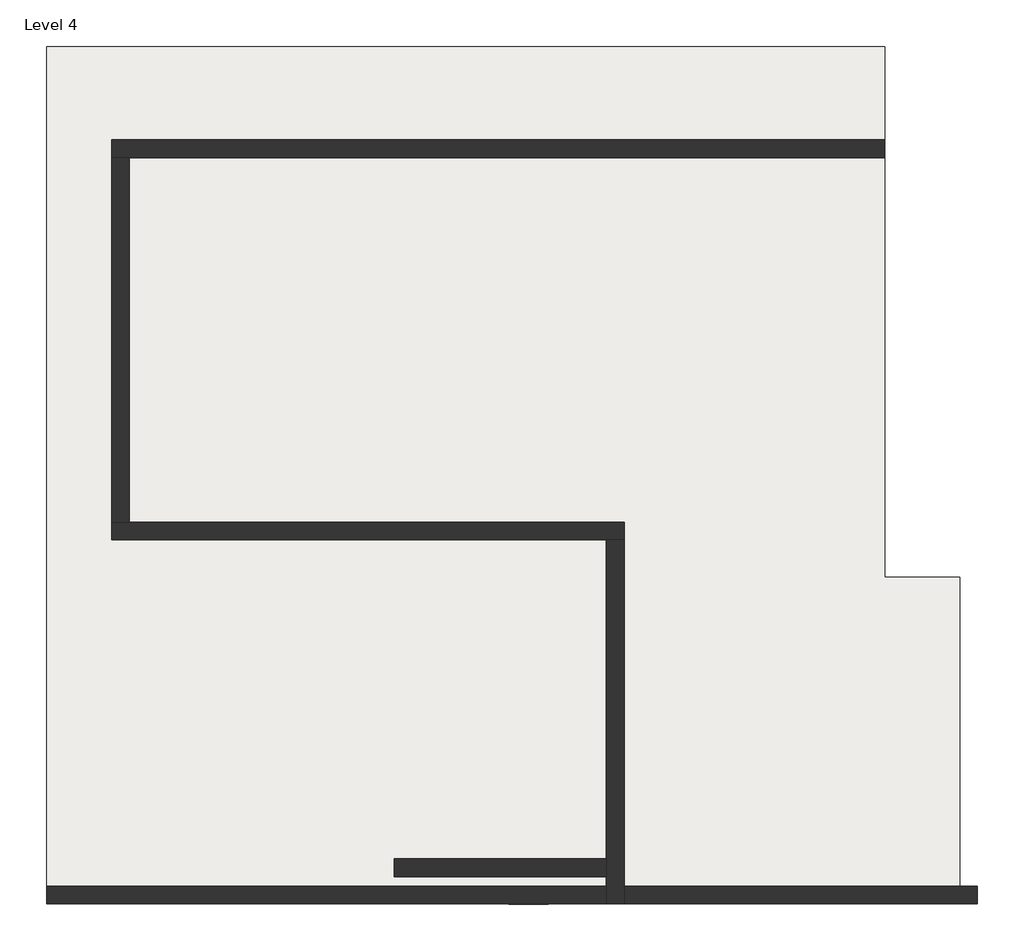
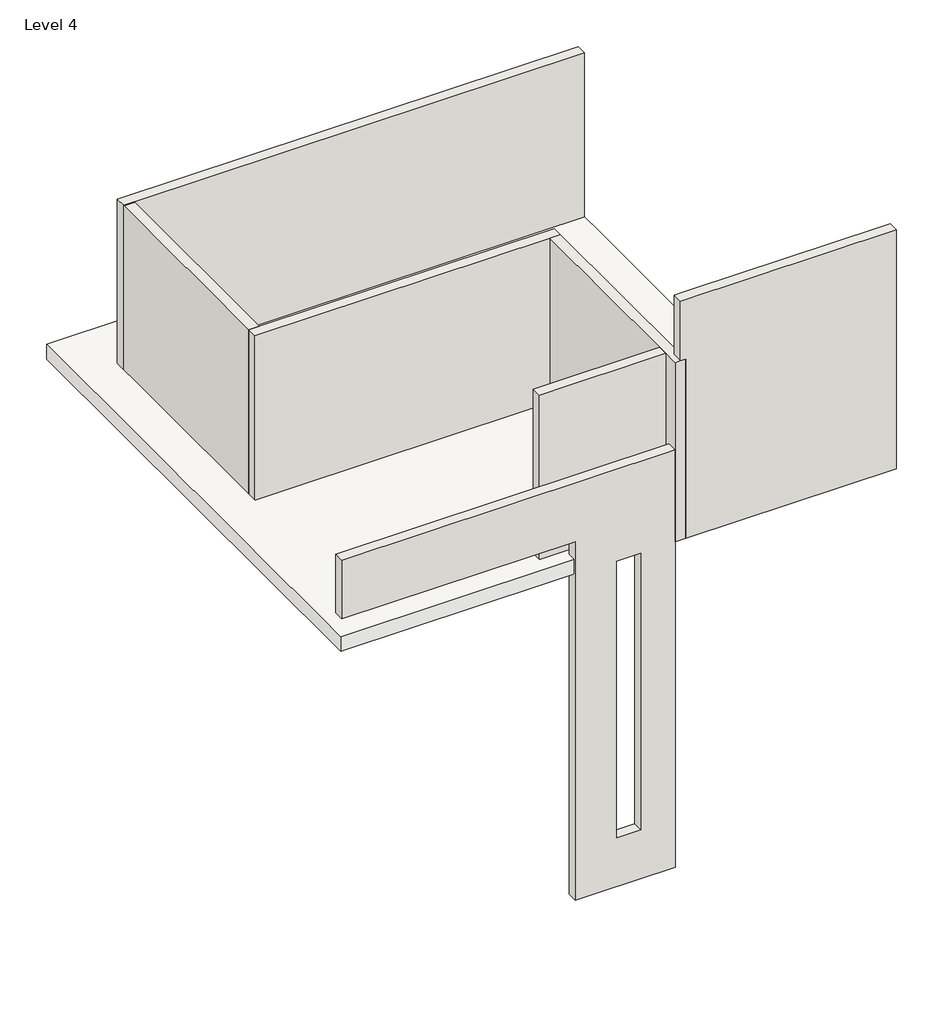
# One storey: 7 walls, 1 roof.
"""IFC4 building model written with IfcOpenShell, lengths in millimetres."""

from ifc_helpers import new_model, si_unit, frame, origin, place, context, project, spatial, polyline, outline, extrude, faceted_brep, element, save

model = new_model("IFC4")

# Units and contexts
model_context = context("Model", 3, world=origin())
ifc_project = project(units=[si_unit("LENGTHUNIT", "METRE", prefix="MILLI")], contexts=[model_context])

# Site, building, storey
site = spatial("IfcSite", under=ifc_project)
building = spatial("IfcBuilding", under=site)
storey = spatial("IfcBuildingStorey", under=building, Name="Level 4", Elevation=10972.8)

# Roof
placement = place(None, origin())
element("IfcRoof", 1, ObjectType="Generic - 12\"", at=placement, inside=storey, context=model_context, shape_type="SweptSolid", body=[
    extrude(outline(polyline([(-10862.1012689, 11214.3911137), (-1224.1821198, 11214.3911137), (-1224.1821198, 5111.80098), (-360.5821198, 5111.80098), (-360.5821198, 1387.3881635), (-10862.1012689, 1387.3881635), (-10862.1012689, 11214.3911137)])), frame((0.0, 0.0, 10972.8), z_axis=(0.0, 0.0, 1.0), x_axis=(1.0, 0.0, 0.0)), (0.0, 0.0, 1.0), 304.8),
])

# Walls
element("IfcWall", 2, ObjectType="Generic - 8\"", at=placement, inside=storey, context=model_context, shape_type="Brep", body=[
    faceted_brep([(-10114.1821198, 9937.80098, 11150.0899101), (-1224.1821198, 9937.80098, 11150.0899101), (-1224.1821198, 9937.80098, 14630.4), (-9910.9821198, 9937.80098, 14630.4), (-10114.1821198, 9937.80098, 14630.4), (-10114.1821198, 10141.00098, 11150.0899101), (-10114.1821198, 10141.00098, 14630.4), (-1224.1821198, 10141.00098, 14630.4), (-1224.1821198, 10141.00098, 11150.0899101)], [[[0, 1, 2, 3, 4]], [[5, 6, 7, 8]], [[1, 0, 5, 8]], [[0, 4, 6, 5]], [[4, 3, 2, 7, 6]], [[1, 8, 7, 2]]]),
])
element("IfcWall", 3, ObjectType="Generic - 8\"", at=placement, inside=storey, context=model_context, shape_type="Brep", body=[
    faceted_brep([(-9910.9821198, 5746.80098, 10972.8), (-9910.9821198, 9937.80098, 10972.8), (-9910.9821198, 9937.80098, 14630.4), (-9910.9821198, 9912.40098, 14630.4), (-9910.9821198, 5746.80098, 14630.4), (-10114.1821198, 5746.80098, 10972.8), (-10114.1821198, 5746.80098, 14630.4), (-10114.1821198, 9912.40098, 14630.4), (-10114.1821198, 9937.80098, 14630.4), (-10114.1821198, 9937.80098, 11150.0899101), (-10114.1821198, 9937.80098, 10972.8)], [[[0, 1, 2, 3, 4]], [[5, 6, 7, 8, 9, 10]], [[1, 0, 5, 10]], [[2, 1, 10, 9, 8]], [[0, 4, 6, 5]], [[3, 2, 8, 7]], [[4, 3, 7, 6]]]),
])
element("IfcWall", 4, ObjectType="Generic - 8\"", at=placement, inside=storey, context=model_context, shape_type="Brep", body=[
    faceted_brep([(-10114.1821198, 5543.60098, 10972.8), (-4424.5821198, 5543.60098, 10972.8), (-4221.3821198, 5543.60098, 10972.8), (-4221.3821198, 5543.60098, 14630.4), (-4424.5821198, 5543.60098, 14630.4), (-10114.1821198, 5543.60098, 14630.4), (-10114.1821198, 5746.80098, 10972.8), (-10114.1821198, 5746.80098, 14630.4), (-9910.9821198, 5746.80098, 14630.4), (-4221.3821198, 5746.80098, 14630.4), (-4221.3821198, 5746.80098, 10972.8), (-9910.9821198, 5746.80098, 10972.8)], [[[0, 1, 2, 3, 4, 5]], [[6, 7, 8, 9, 10, 11]], [[2, 1, 0, 6, 11, 10]], [[3, 2, 10, 9]], [[0, 5, 7, 6]], [[5, 4, 3, 9, 8, 7]]]),
])
element("IfcWall", 5, ObjectType="Generic - 8\"", at=placement, inside=storey, context=model_context, shape_type="Brep", body=[
    faceted_brep([(-4424.5821198, 5543.60098, 10972.8), (-4424.5821198, 1872.9280349, 10972.8), (-4424.5821198, 1669.7280349, 10972.8), (-4424.5821198, 1355.2652184, 10972.8), (-4424.5821198, 1355.2652184, 12853.3343926), (-4424.5821198, 1355.2652184, 14630.4), (-4424.5821198, 1669.7280349, 14630.4), (-4424.5821198, 1872.9280349, 14630.4), (-4424.5821198, 5543.60098, 14630.4), (-4221.3821198, 5543.60098, 10972.8), (-4221.3821198, 5543.60098, 14630.4), (-4221.3821198, 1558.4652184, 14630.4), (-4221.3821198, 1549.45098, 14630.4), (-4221.3821198, 1355.2652184, 14630.4), (-4221.3821198, 1355.2652184, 10972.8), (-4221.3821198, 1558.4652184, 10972.8), (-4322.9821198, 1355.2652184, 14630.4)], [[[0, 1, 2, 3, 4, 5, 6, 7, 8]], [[9, 10, 11, 12, 13, 14, 15]], [[3, 2, 1, 0, 9, 15, 14]], [[0, 8, 10, 9]], [[8, 7, 6, 5, 16, 13, 12, 11, 10]], [[3, 14, 13, 16, 5, 4]]]),
])
element("IfcWall", 6, ObjectType="Generic - 8\"", at=placement, inside=storey, context=model_context, shape_type="Brep", body=[
    faceted_brep([(-10858.7268197, 1355.2652184, 11656.9312703), (-6354.9821198, 1355.2652184, 11656.9312703), (-6354.9821198, 1355.2652184, 7084.9312703), (-6354.9821198, 1355.2652184, 4341.7312703), (-5949.9629707, 1355.2652184, 4341.7312703), (-4424.5821198, 1355.2652184, 4341.7312703), (-4424.5821198, 1355.2652184, 10972.8), (-4424.5821198, 1355.2652184, 12853.3343926), (-10858.7268197, 1355.2652184, 12853.3343926), (-5090.6416943, 1355.2652184, 10972.8), (-5090.6416943, 1355.2652184, 5334.0), (-5547.8416943, 1355.2652184, 5334.0), (-5547.8416943, 1355.2652184, 10972.8), (-10858.7268197, 1558.4652184, 11656.9312703), (-10858.7268197, 1558.4652184, 12853.3343926), (-4424.5821198, 1558.4652184, 12853.3343926), (-4424.5821198, 1558.4652184, 4341.7312703), (-5949.9629707, 1558.4652184, 4341.7312703), (-6354.9821198, 1558.4652184, 4341.7312703), (-6354.9821198, 1558.4652184, 7084.9312703), (-6354.9821198, 1558.4652184, 11656.9312703), (-5090.6416943, 1558.4652184, 10972.8), (-5547.8416943, 1558.4652184, 10972.8), (-5547.8416943, 1558.4652184, 5334.0), (-5090.6416943, 1558.4652184, 5334.0)], [[[0, 1, 2, 3, 4, 5, 6, 7, 8], [9, 10, 11, 12]], [[13, 14, 15, 16, 17, 18, 19, 20], [21, 22, 23, 24]], [[7, 6, 5, 16, 15]], [[5, 4, 3, 18, 17, 16]], [[0, 8, 14, 13]], [[1, 0, 13, 20]], [[1, 20, 19, 18, 3, 2]], [[8, 7, 15, 14]], [[10, 9, 21, 24]], [[11, 10, 24, 23]], [[12, 11, 23, 22]], [[9, 12, 22, 21]]]),
])
element("IfcWall", 7, ObjectType="Generic - 8\"", at=placement, inside=storey, context=model_context, shape_type="Brep", body=[
    faceted_brep([(-4221.3821198, 1355.2652184, 10972.8), (-157.3821198, 1355.2652184, 10972.8), (-157.3821198, 1355.2652184, 15849.6), (-4322.9821198, 1355.2652184, 15849.6), (-4322.9821198, 1355.2652184, 14630.4), (-4221.3821198, 1355.2652184, 14630.4), (-4221.3821198, 1558.4652184, 10972.8), (-4221.3821198, 1558.4652184, 14630.4), (-4322.9821198, 1558.4652184, 14630.4), (-4322.9821198, 1558.4652184, 15849.6), (-4221.3821198, 1558.4652184, 15849.6), (-4018.1821198, 1558.4652184, 15849.6), (-360.5821198, 1558.4652184, 15849.6), (-157.3821198, 1558.4652184, 15849.6), (-157.3821198, 1558.4652184, 10972.8), (-360.5821198, 1558.4652184, 10972.8), (-157.3821198, 1447.4780349, 10972.8)], [[[0, 1, 2, 3, 4, 5]], [[6, 7, 8, 9, 10, 11, 12, 13, 14, 15]], [[1, 0, 6, 15, 14, 16]], [[3, 2, 13, 12, 11, 10, 9]], [[4, 3, 9, 8]], [[4, 8, 7, 5]], [[0, 5, 7, 6]], [[2, 1, 16, 14, 13]]]),
])
element("IfcWall", 8, ObjectType="Generic - 8\"", at=placement, inside=storey, context=model_context, shape_type="SweptSolid", body=[
    extrude(outline(polyline([(-6862.9821198, 1872.9280349), (-4424.5821198, 1872.9280349), (-4424.5821198, 1669.7280349), (-6862.9821198, 1669.7280349), (-6862.9821198, 1872.9280349)])), frame((0.0, 0.0, 10972.8), z_axis=(0.0, 0.0, 1.0), x_axis=(1.0, 0.0, 0.0)), (0.0, 0.0, 1.0), 3657.6),
])

save(model, "model.ifc")

# Revit data of these elements
# Type "Generic - 12\""
#   Assembly Code = "B1020"
#   Layers, outside or top first: 1' - 0" no material (function 1)
# Type "Generic - 8\""
#   Assembly Code = "B2010"
#   Layers, outside or top first: 0' - 8" no material (function 1)
# Element 1 (IfcRoof, "Generic - 12\"")
#   built-in parameter 1001705 = 37 (stored number, unit not read)
#   built-in parameter 1001710 = 33615
#   Phase Created = New Construction
#   Materials on its faces: "Default Roof"
# Element 2 (IfcWall, "Generic - 8\"")
#   built-in parameter 1001111 = 0' - 6.97992"
#   Top Offset = 0' - 0"
#   Base Offset = 0' - 6.97992"
#   Unconnected Height = 12' - 4"
#   wall height = 12' - 4"
#   Phase Created = New Construction
#   Base Constraint = Level 4
#   Materials on its faces: "Default Wall"
# Elements 3, 4 (IfcWall, "Generic - 8\"")
#   Top Offset = 0' - 0"
#   Base Offset = 0' - 0"
#   Unconnected Height = 12' - 0"
#   wall height = 12' - 0"
#   Phase Created = New Construction
#   Base Constraint = Level 4
#   Materials on its faces: "Default Wall"
# Elements 5, 8 (IfcWall, "Generic - 8\"")
#   Top Offset = 0' - 0"
#   Base Offset = 0' - 0"
#   Unconnected Height = 12' - 0"
#   wall height = 12' - 0"
#   Phase Created = New Construction
#   Base Constraint = Level 4
#   Materials on its faces: "Default Wall", "Tile, Porcelain, 4in"
# Element 6 (IfcWall, "Generic - 8\"")
#   built-in parameter 1001111 = -21' - 9.0657"
#   Top Offset = 0' - 0"
#   Base Offset = -21' - 9.0657"
#   Unconnected Height = 28' - 11.10249"
#   wall height = 28' - 11.10249"
#   Phase Created = New Construction
#   Base Constraint = Level 4
#   Materials on its faces: "Default Wall", "Brick, Common"
# Element 7 (IfcWall, "Generic - 8\"")
#   Top Offset = 0' - 0"
#   Base Offset = 0' - 0"
#   Unconnected Height = 16' - 0"
#   wall height = 16' - 0"
#   Phase Created = New Construction
#   Base Constraint = Level 4
#   Materials on its faces: "Default Wall", "Tile, Porcelain, 4in"
# Materials
#   "Default Roof": colour RGB 88 101 114, transparency 0
#   "Default Wall": colour RGB 128 128 128, transparency 0
#   "Tile, Porcelain, 4in": class "Generic", colour RGB 89 87 158, transparency 0, Description = "Porcelain tile, 4\", white", Cost = 0
#   "Brick, Common": class "Masonry", colour RGB 170 98 104, transparency 0, Description = "Common brick", Cost = 0
